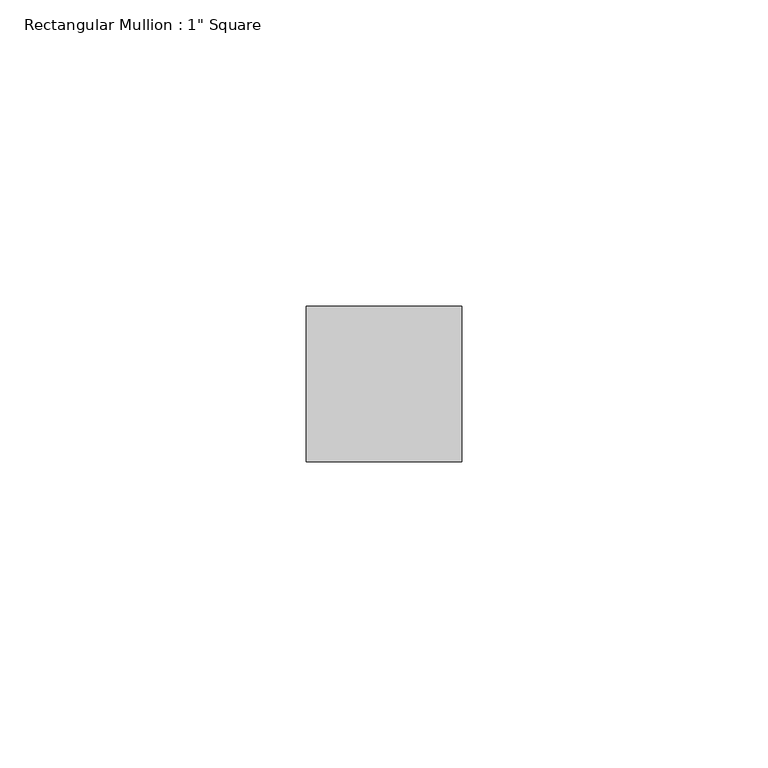
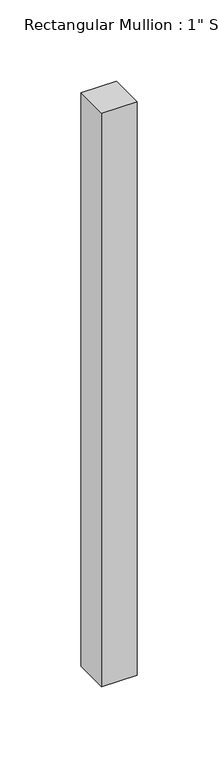
"""IFC4 building model written with IfcOpenShell, lengths in millimetres: member geometry."""

from ifc_helpers import new_model, si_unit, frame, origin, place, context, project, spatial, polyline, outline, extrude, source, transform, mapped, element, save


def member_0e6c94ff(model_context):
    return source(origin(), model_context, "Body", "SweptSolid", [
        extrude(outline(polyline([(0.0, 12.7), (0.0, -12.7), (-25.4, -12.7), (-25.4, 12.7), (0.0, 12.7)])), frame((0.0, 0.0, -431.8), z_axis=(0.0, 0.0, 1.0), x_axis=(1.0, 0.0, 0.0)), (0.0, 0.0, 1.0), 431.8),
    ])


if __name__ == "__main__":
    model = new_model("IFC4")
    model_context = context("Model", 3, world=origin())
    ifc_project = project(units=[si_unit("LENGTHUNIT", "METRE", prefix="MILLI")], contexts=[model_context])
    site = spatial("IfcSite", under=ifc_project)
    building = spatial("IfcBuilding", under=site)
    placement = place(None, origin())
    member_shape = member_0e6c94ff(model_context)
    element("IfcMember", 1, ObjectType="Rectangular Mullion : 1\" Square", at=placement, inside=building, context=model_context, shape_type="MappedRepresentation", body=[
        mapped(member_shape, transform((0.0, 0.0, 0.0), x_axis=(1.0, 0.0, 0.0), y_axis=(0.0, 1.0, 0.0), z_axis=(0.0, 0.0, 1.0))),
    ])
    save(model, "model.ifc")

# Revit data of these elements
# Type "Rectangular Mullion : 1\" Square"
#   built-in parameter 1007304 = 0.0833333 (stored number, unit not read)
#   built-in parameter 1007301 = 0.0416667 (stored number, unit not read)
#   built-in parameter 1007300 = 0.0416667 (stored number, unit not read)
# Element 1 (IfcMember, "Rectangular Mullion : 1\" Square")
#   Materials on its faces: "Aluminum"
# Materials
#   "Aluminum": class "Metal", colour RGB 247 247 247, transparency 0, Description = "Aluminum 6061", Cost = 0
